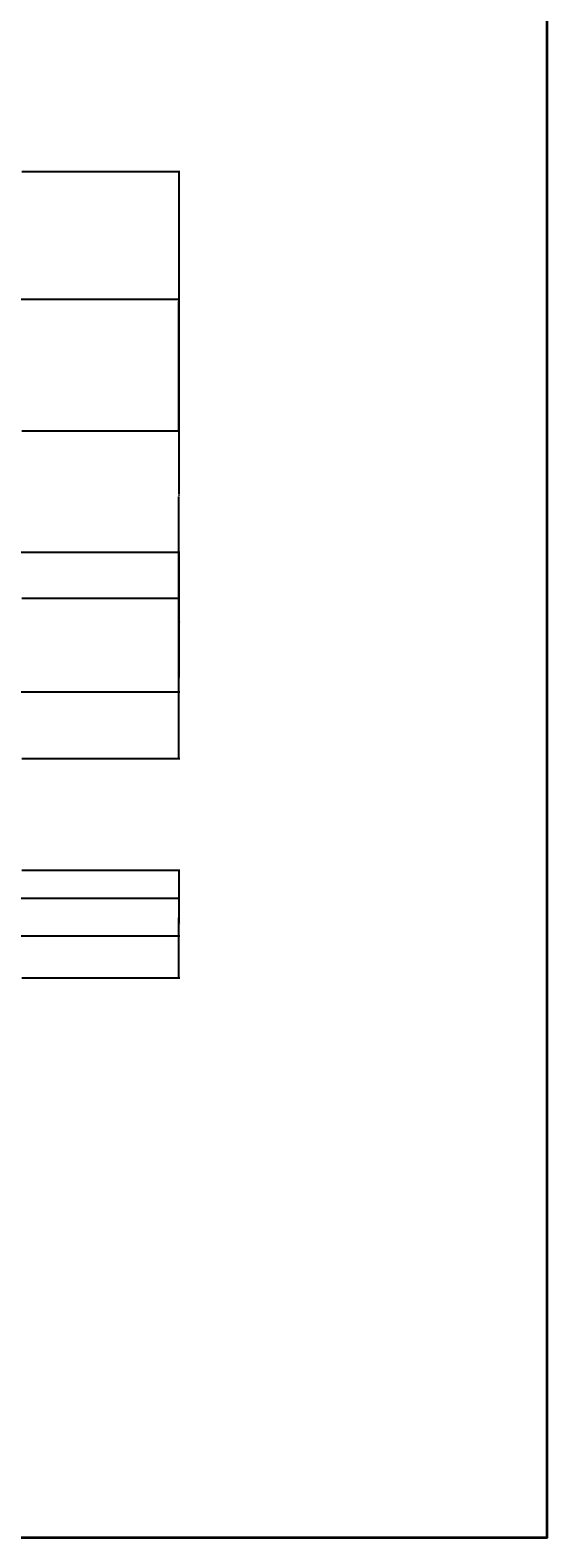
# Model space of a CAD drawing. Units: inches. Extents: x 2310 to 2937, y 1113 to 2410.
# Tile 15 of 23: x 2826 to 2937, y 1616 to 1940. Entities that reach past the tile are written whole.
import ezdxf

# ---------------------------------------------------------------- set-up
doc = ezdxf.new("R2010")
doc.units = ezdxf.units.IN
doc.layers.add('A-ANNO-DIMS', color=2, linetype='Continuous', lineweight=18)
doc.layers.add('A-ANNO-TTLB', color=7, linetype='Continuous', lineweight=35)
doc.styles.get("Standard").update_dxf_attribs({"font": 'arial.ttf'})
doc.dimstyles.get("Standard").update_dxf_attribs({"dimtxt": 0.18, "dimasz": 0.18, "dimexe": 0.18, "dimexo": 0.0625, "dimgap": 0.09, "dimtad": 0, "dimtih": 1, "dimtoh": 1, "dimdec": 4, "dimzin": 0, "dimdsep": 46, "dimtxsty": 'Standard', "dimcen": 0.09, "dimadec": 0, "dimazin": 0, "dimtfac": 1, "dimtdec": 4, "dimtofl": 0, "dimtmove": 0, "dimatfit": 3, "dimfxl": 1, "dimtolj": 1, "dimtzin": 0, "dimarcsym": 0})

# ---------------------------------------------------------------- blocks, each defined once
blk = doc.blocks.new('*D45')
at = {"layer": 'A-ANNO-DIMS', "color": 0, "lineweight": -2, "transparency": 16777216}
for p, q in [((2824.05, 1759.67), (2858.02, 1759.67)), ((2857.84, 1759.49), (2857.84, 1748.27)), ((2857.84, 1736.69), (2857.84, 1747.91)), ((2824.05, 1736.51), (2858.02, 1736.51))]:
    blk.add_line(p, q, dxfattribs=at)
at = {"layer": 'A-ANNO-DIMS', "color": 0, "transparency": 16777216}
for points in [[(2857.81, 1759.49), (2857.87, 1759.49), (2857.84, 1759.67)], [(2857.81, 1736.69), (2857.87, 1736.69), (2857.84, 1736.51)]]:
    blk.add_solid(points, dxfattribs=at)
at = {"layer": 'Defpoints', "color": 0, "transparency": 16777216}
for p in [(2823.99, 1759.67), (2857.84, 1759.67), (2823.99, 1736.51)]:
    blk.add_point(p, dxfattribs=at)
at = {"layer": 'A-ANNO-DIMS', "color": 0, "transparency": 16777216, "insert": (2857.84, 1748.09), "char_height": 0.18, "attachment_point": 5}
blk.add_mtext('\\A1;23.154', dxfattribs=at)
blk = doc.blocks.new('*D46')
at = {"layer": 'A-ANNO-DIMS', "color": 0, "lineweight": -2, "transparency": 16777216}
for p, q in [((2824.05, 1818.17), (2858.02, 1818.17)), ((2857.84, 1817.99), (2857.84, 1801.1)), ((2857.84, 1783.85), (2857.84, 1800.74)), ((2824.05, 1783.67), (2858.02, 1783.67))]:
    blk.add_line(p, q, dxfattribs=at)
at = {"layer": 'A-ANNO-DIMS', "color": 0, "transparency": 16777216}
for points in [[(2857.81, 1817.99), (2857.87, 1817.99), (2857.84, 1818.17)], [(2857.81, 1783.85), (2857.87, 1783.85), (2857.84, 1783.67)]]:
    blk.add_solid(points, dxfattribs=at)
at = {"layer": 'Defpoints', "color": 0, "transparency": 16777216}
for p in [(2823.99, 1818.17), (2857.84, 1818.17), (2823.99, 1783.67)]:
    blk.add_point(p, dxfattribs=at)
at = {"layer": 'A-ANNO-DIMS', "color": 0, "transparency": 16777216, "insert": (2857.84, 1800.92), "char_height": 0.18, "attachment_point": 5}
blk.add_mtext('\\A1;34.5', dxfattribs=at)
blk = doc.blocks.new('*D47')
at = {"layer": 'A-ANNO-DIMS', "color": 0, "lineweight": -2, "transparency": 16777216}
for p, q in [((2824.05, 1909.98), (2858.02, 1909.98)), ((2857.84, 1909.8), (2857.84, 1882.26)), ((2857.84, 1854.35), (2857.84, 1881.89)), ((2824.05, 1854.17), (2858.02, 1854.17))]:
    blk.add_line(p, q, dxfattribs=at)
at = {"layer": 'A-ANNO-DIMS', "color": 0, "transparency": 16777216}
for points in [[(2857.81, 1909.8), (2857.87, 1909.8), (2857.84, 1909.98)], [(2857.81, 1854.35), (2857.87, 1854.35), (2857.84, 1854.17)]]:
    blk.add_solid(points, dxfattribs=at)
at = {"layer": 'Defpoints', "color": 0, "transparency": 16777216}
for p in [(2823.99, 1909.98), (2857.84, 1909.98), (2823.99, 1854.17)]:
    blk.add_point(p, dxfattribs=at)
at = {"layer": 'A-ANNO-DIMS', "color": 0, "transparency": 16777216, "insert": (2857.84, 1882.07), "char_height": 0.18, "attachment_point": 5}
blk.add_mtext('\\A1;55.81', dxfattribs=at)
blk = doc.blocks.new('*D55')
at = {"layer": 'A-ANNO-DIMS', "color": 0, "lineweight": -2, "transparency": 16777216}
for p, q in [((2403.55, 1753.64), (2858.02, 1753.64)), ((2857.84, 1753.46), (2857.84, 1749.76)), ((2857.84, 1745.69), (2857.84, 1749.4)), ((2403.55, 1745.51), (2858.02, 1745.51))]:
    blk.add_line(p, q, dxfattribs=at)
at = {"layer": 'A-ANNO-DIMS', "color": 0, "transparency": 16777216}
for points in [[(2857.81, 1753.46), (2857.87, 1753.46), (2857.84, 1753.64)], [(2857.81, 1745.69), (2857.87, 1745.69), (2857.84, 1745.51)]]:
    blk.add_solid(points, dxfattribs=at)
at = {"layer": 'Defpoints', "color": 0, "transparency": 16777216}
for p in [(2403.49, 1753.64), (2857.84, 1753.64), (2403.49, 1745.51)]:
    blk.add_point(p, dxfattribs=at)
at = {"layer": 'A-ANNO-DIMS', "color": 0, "transparency": 16777216, "insert": (2857.84, 1749.58), "char_height": 0.18, "attachment_point": 5}
blk.add_mtext('\\A1;8.127', dxfattribs=at)
blk = doc.blocks.new('*D56')
at = {"layer": 'A-ANNO-DIMS', "color": 0, "lineweight": -2, "transparency": 16777216}
for p, q in [((2403.55, 1828.04), (2858.02, 1828.04)), ((2857.84, 1827.86), (2857.84, 1813.21)), ((2857.84, 1798.19), (2857.84, 1812.85)), ((2403.55, 1798.01), (2858.02, 1798.01))]:
    blk.add_line(p, q, dxfattribs=at)
at = {"layer": 'A-ANNO-DIMS', "color": 0, "transparency": 16777216}
for points in [[(2857.81, 1827.86), (2857.87, 1827.86), (2857.84, 1828.04)], [(2857.81, 1798.19), (2857.87, 1798.19), (2857.84, 1798.01)]]:
    blk.add_solid(points, dxfattribs=at)
at = {"layer": 'Defpoints', "color": 0, "transparency": 16777216}
for p in [(2403.49, 1828.04), (2857.84, 1828.04), (2403.49, 1798.01)]:
    blk.add_point(p, dxfattribs=at)
at = {"layer": 'A-ANNO-DIMS', "color": 0, "transparency": 16777216, "insert": (2857.84, 1813.03), "char_height": 0.18, "attachment_point": 5}
blk.add_mtext('\\A1;30.03', dxfattribs=at)
blk = doc.blocks.new('*D58')
at = {"layer": 'A-ANNO-DIMS', "color": 0, "lineweight": -2, "transparency": 16777216}
for p, q in [((2475.55, 1882.51), (2858.02, 1882.51)), ((2857.84, 1882.33), (2857.84, 1840.45)), ((2857.84, 1798.19), (2857.84, 1840.08)), ((2475.55, 1798.01), (2858.02, 1798.01))]:
    blk.add_line(p, q, dxfattribs=at)
at = {"layer": 'A-ANNO-DIMS', "color": 0, "transparency": 16777216}
for points in [[(2857.81, 1882.33), (2857.87, 1882.33), (2857.84, 1882.51)], [(2857.81, 1798.19), (2857.87, 1798.19), (2857.84, 1798.01)]]:
    blk.add_solid(points, dxfattribs=at)
at = {"layer": 'Defpoints', "color": 0, "transparency": 16777216}
for p in [(2475.49, 1882.51), (2857.84, 1882.51), (2475.49, 1798.01)]:
    blk.add_point(p, dxfattribs=at)
at = {"layer": 'A-ANNO-DIMS', "color": 0, "transparency": 16777216, "insert": (2857.84, 1840.26), "char_height": 0.18, "attachment_point": 5}
blk.add_mtext('\\A1;84.5', dxfattribs=at)

msp = doc.modelspace()

# ---------------------------------------------------------------- linework, layer by layer
at = {"layer": 'A-ANNO-TTLB'}
msp.add_lwpolyline([(2310.2498, 2409.8427), (2937.0534, 2409.8427), (2937.0534, 1616.036), (2310.2498, 1616.036)], close=True, dxfattribs=at)

# ---------------------------------------------------------------- dimensions: what is measured, and where the dimension line sits
at = {"layer": 'A-ANNO-DIMS'}
for base, p1, p2, override, picture, middle in [((2857.8359, 1909.9784), (2823.9859, 1854.1704), (2823.9859, 1909.9784), {"dimdec": 2, "dimlfac": 1, "dimrnd": 0, "dimzin": 0, "dimdsep": 46, "dimlunit": 2}, '*D47', (2857.8359, 1882.0744)), ((2857.8359, 1882.5139), (2475.4859, 1798.0139), (2475.4859, 1882.5139), {"dimdec": 1, "dimlfac": 1, "dimrnd": 0, "dimzin": 0, "dimdsep": 46, "dimlunit": 2}, '*D58', (2857.8359, 1840.2639)), ((2857.8359, 1828.0433), (2403.4859, 1798.0139), (2403.4859, 1828.0433), {"dimdec": 2, "dimlfac": 1, "dimrnd": 0, "dimzin": 0, "dimdsep": 46, "dimlunit": 2}, '*D56', (2857.8359, 1813.0286)), ((2857.8359, 1818.1704), (2823.9859, 1783.6684), (2823.9859, 1818.1704), {"dimdec": 1, "dimlfac": 1, "dimrnd": 0, "dimzin": 0, "dimdsep": 46, "dimlunit": 2}, '*D46', (2857.8359, 1800.9194)), ((2857.83594, 1759.66842), (2823.98594, 1736.51394), (2823.98594, 1759.66842), {"dimdec": 3, "dimlfac": 1, "dimrnd": 0, "dimzin": 0, "dimdsep": 46, "dimlunit": 2}, '*D45', (2857.83594, 1748.09118)), ((2857.8359, 1753.6409), (2403.4859, 1745.5139), (2403.4859, 1753.6409), {"dimdec": 3, "dimlfac": 1, "dimrnd": 0, "dimzin": 0, "dimdsep": 46, "dimlunit": 2}, '*D55', (2857.8359, 1749.5774))]:
    dim = msp.add_linear_dim(base=base, p1=p1, p2=p2, angle=90, dimstyle='Standard', override=override, dxfattribs=at)
    dim.commit()
    dim.dimension.update_dxf_attribs({"geometry": picture, "text_midpoint": middle})

doc.saveas('drawing.dxf')
